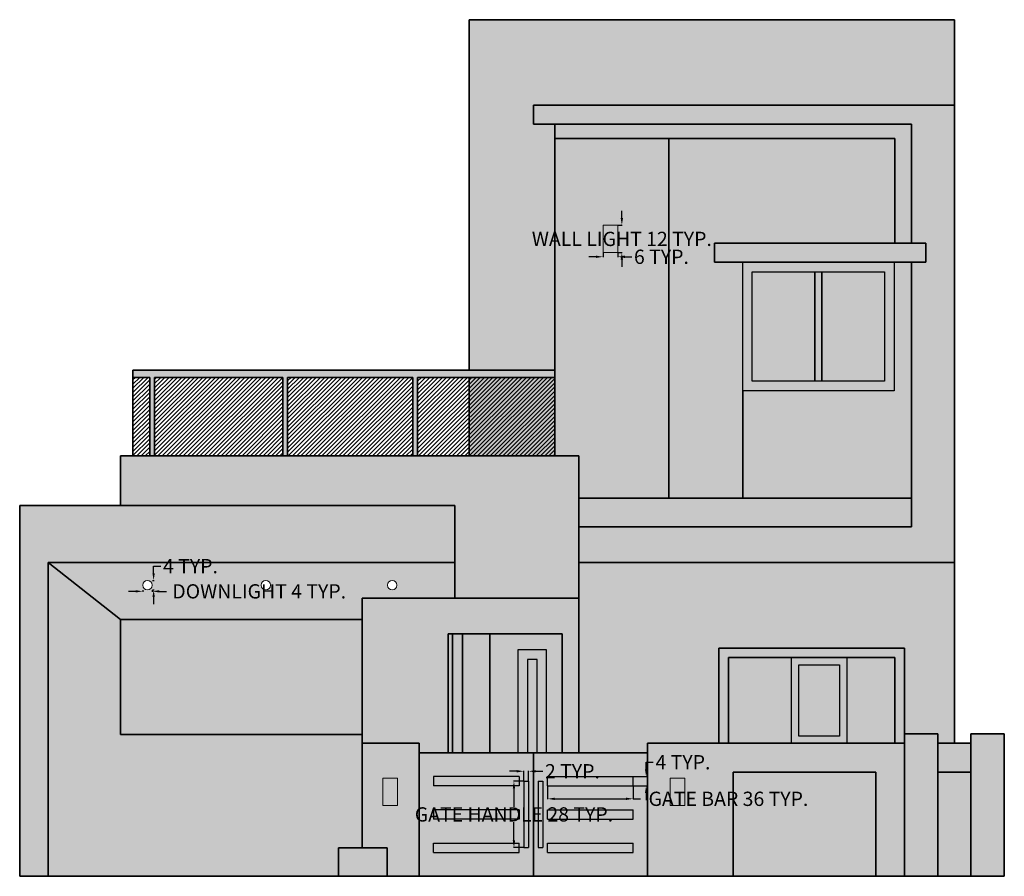
# Model space of a CAD drawing. Units: inches. Extents: x 25 to 439, y 12 to 373.
import ezdxf

# ---------------------------------------------------------------- set-up
doc = ezdxf.new("R2010")
doc.units = ezdxf.units.IN
doc.header["$MEASUREMENT"] = 0
for name, color, linetype, lineweight in [('A-ANNO-DIMS', 2, 'Continuous', 18), ('A-DOOR', 3, 'Continuous', 25), ('A-ELEV', 7, 'Continuous', 35), ('A-ELEV-PATT', 8, 'Continuous', 13), ('A-GLAZ', 4, 'Continuous', 25), ('E-LITE', 2, 'Continuous', 18)]:
    doc.layers.add(name, color=color, linetype=linetype, lineweight=lineweight)
doc.styles.get("Standard").update_dxf_attribs({"font": 'arial.ttf'})
doc.dimstyles.get("Standard").update_dxf_attribs({"dimtxt": 6, "dimasz": 3, "dimexe": 0.18, "dimexo": 0.0625, "dimgap": 0.09, "dimtad": 0, "dimtih": 1, "dimtoh": 1, "dimdec": 0, "dimzin": 0, "dimdsep": 46, "dimlunit": 3, "dimtxsty": 'Standard', "dimcen": 0.09, "dimadec": 0, "dimazin": 0, "dimtfac": 1, "dimtdec": 0, "dimtofl": 0, "dimtmove": 0, "dimatfit": 3, "dimfxl": 1, "dimtolj": 1, "dimtzin": 0, "dimarcsym": 0})

# ---------------------------------------------------------------- blocks, each defined once
blk = doc.blocks.new('GATE-BAR')
for p, q in [((0, 0), (0, 4)), ((0, 4), (36, 4)), ((36, 0), (36, 4)), ((0, 0), (36, 0))]:
    blk.add_line(p, q)
blk = doc.blocks.new('GATE-HANDLE')
for p, q in [((0, 27.93), (0, 0)), ((0, 27.93), (2, 27.93)), ((2, 27.93), (2, 0)), ((0, 0), (2, 0))]:
    blk.add_line(p, q)
blk = doc.blocks.new('WALL-LIGHT')
blk.add_lwpolyline([(0, 11.58), (6.15, 11.58), (6.15, 0), (0, 0)], close=True)
blk = doc.blocks.new('LIGHT-DOWN')
blk.add_circle((2, 2), 2)
blk = doc.blocks.new('*D5')
at = {"layer": 'A-ANNO-DIMS', "color": 0, "lineweight": -2, "transparency": 16777216}
for p, q in [((246.85, 50.12), (246.85, 44.6)), ((282.85, 50.12), (282.85, 44.6)), ((249.85, 44.78), (279.85, 44.78)), ((282.85, 44.78), (285.85, 44.78))]:
    blk.add_line(p, q, dxfattribs=at)
at = {"layer": 'A-ANNO-DIMS', "color": 0, "transparency": 16777216}
for points in [[(249.85, 45.28), (249.85, 44.28), (246.85, 44.78)], [(279.85, 45.28), (279.85, 44.28), (282.85, 44.78)]]:
    blk.add_solid(points, dxfattribs=at)
at = {"layer": 'Defpoints', "color": 0, "transparency": 16777216}
for p in [(246.85, 50.18), (282.85, 50.18), (282.85, 44.78)]:
    blk.add_point(p, dxfattribs=at)
at = {"layer": 'A-ANNO-DIMS', "color": 0, "transparency": 16777216, "insert": (322.86, 44.78), "char_height": 6, "attachment_point": 5}
blk.add_mtext('\\A1;GATE BAR 36 TYP.', dxfattribs=at)
blk = doc.blocks.new('*D6')
at = {"layer": 'A-ANNO-DIMS', "color": 0, "lineweight": -2, "transparency": 16777216}
for p, q in [((288.25, 57.18), (288.25, 60.18)), ((288.25, 60.18), (291.25, 60.18)), ((282.92, 54.18), (288.43, 54.18)), ((282.92, 50.18), (288.43, 50.18)), ((288.25, 47.18), (288.25, 44.18))]:
    blk.add_line(p, q, dxfattribs=at)
at = {"layer": 'A-ANNO-DIMS', "color": 0, "transparency": 16777216}
for points in [[(287.75, 57.18), (288.75, 57.18), (288.25, 54.18)], [(287.75, 47.18), (288.75, 47.18), (288.25, 50.18)]]:
    blk.add_solid(points, dxfattribs=at)
at = {"layer": 'Defpoints', "color": 0, "transparency": 16777216}
for p in [(282.85, 54.18), (288.25, 54.18), (282.85, 50.18)]:
    blk.add_point(p, dxfattribs=at)
at = {"layer": 'A-ANNO-DIMS', "color": 0, "transparency": 16777216, "insert": (303.74, 60.18), "char_height": 6, "attachment_point": 5}
blk.add_mtext('\\A1;4 TYP.', dxfattribs=at)
blk = doc.blocks.new('*D7')
at = {"layer": 'A-ANNO-DIMS', "color": 0, "lineweight": -2, "transparency": 16777216}
for p, q in [((278.04, 289.09), (278.04, 292.09)), ((276.37, 286.09), (278.22, 286.09)), ((276.37, 274.51), (278.22, 274.51)), ((278.04, 271.51), (278.04, 268.51))]:
    blk.add_line(p, q, dxfattribs=at)
at = {"layer": 'A-ANNO-DIMS', "color": 0, "transparency": 16777216}
for points in [[(277.54, 289.09), (278.54, 289.09), (278.04, 286.09)], [(277.54, 271.51), (278.54, 271.51), (278.04, 274.51)]]:
    blk.add_solid(points, dxfattribs=at)
at = {"layer": 'Defpoints', "color": 0, "transparency": 16777216}
for p in [(276.31, 286.09), (278.04, 286.09), (276.31, 274.51)]:
    blk.add_point(p, dxfattribs=at)
at = {"layer": 'A-ANNO-DIMS', "color": 0, "transparency": 16777216, "insert": (278.04, 280.3), "char_height": 6, "attachment_point": 5}
blk.add_mtext('\\A1;WALL LIGHT 12 TYP.', dxfattribs=at)
blk = doc.blocks.new('*D8')
at = {"layer": 'A-ANNO-DIMS', "color": 0, "lineweight": -2, "transparency": 16777216}
for p, q in [((270.16, 274.45), (270.16, 272.6)), ((276.31, 274.45), (276.31, 272.6)), ((267.16, 272.78), (264.16, 272.78)), ((279.31, 272.78), (282.31, 272.78))]:
    blk.add_line(p, q, dxfattribs=at)
at = {"layer": 'A-ANNO-DIMS', "color": 0, "transparency": 16777216}
for points in [[(267.16, 273.28), (267.16, 272.28), (270.16, 272.78)], [(279.31, 273.28), (279.31, 272.28), (276.31, 272.78)]]:
    blk.add_solid(points, dxfattribs=at)
at = {"layer": 'Defpoints', "color": 0, "transparency": 16777216}
for p in [(270.16, 274.51), (276.31, 274.51), (276.31, 272.78)]:
    blk.add_point(p, dxfattribs=at)
at = {"layer": 'A-ANNO-DIMS', "color": 0, "transparency": 16777216, "insert": (294.68, 272.78), "char_height": 6, "attachment_point": 5}
blk.add_mtext('\\A1;6 TYP.', dxfattribs=at)
blk = doc.blocks.new('*D9')
at = {"layer": 'A-ANNO-DIMS', "color": 0, "lineweight": -2, "transparency": 16777216}
for p, q in [((76.57, 132.59), (76.57, 131.87)), ((80.57, 132.59), (80.57, 131.87)), ((73.57, 132.05), (70.57, 132.05)), ((83.57, 132.05), (86.57, 132.05))]:
    blk.add_line(p, q, dxfattribs=at)
at = {"layer": 'A-ANNO-DIMS', "color": 0, "transparency": 16777216}
for points in [[(73.57, 132.55), (73.57, 131.55), (76.57, 132.05)], [(83.57, 132.55), (83.57, 131.55), (80.57, 132.05)]]:
    blk.add_solid(points, dxfattribs=at)
at = {"layer": 'Defpoints', "color": 0, "transparency": 16777216}
for p in [(76.57, 132.65), (80.57, 132.65), (80.57, 132.05)]:
    blk.add_point(p, dxfattribs=at)
at = {"layer": 'A-ANNO-DIMS', "color": 0, "transparency": 16777216, "insert": (125.56, 132.05), "char_height": 6, "attachment_point": 5}
blk.add_mtext('\\A1;DOWNLIGHT 4 TYP.', dxfattribs=at)
blk = doc.blocks.new('*D10')
at = {"layer": 'A-ANNO-DIMS', "color": 0, "lineweight": -2, "transparency": 16777216}
for p, q in [((81.17, 139.65), (81.17, 142.65)), ((81.17, 142.65), (84.17, 142.65)), ((80.63, 136.65), (81.35, 136.65)), ((80.63, 132.65), (81.35, 132.65)), ((81.17, 129.65), (81.17, 126.65))]:
    blk.add_line(p, q, dxfattribs=at)
at = {"layer": 'A-ANNO-DIMS', "color": 0, "transparency": 16777216}
for points in [[(80.67, 139.65), (81.67, 139.65), (81.17, 136.65)], [(80.67, 129.65), (81.67, 129.65), (81.17, 132.65)]]:
    blk.add_solid(points, dxfattribs=at)
at = {"layer": 'Defpoints', "color": 0, "transparency": 16777216}
for p in [(80.57, 136.65), (81.17, 136.65), (80.57, 132.65)]:
    blk.add_point(p, dxfattribs=at)
at = {"layer": 'A-ANNO-DIMS', "color": 0, "transparency": 16777216, "insert": (96.66, 142.65), "char_height": 6, "attachment_point": 5}
blk.add_mtext('\\A1;4 TYP.', dxfattribs=at)
blk = doc.blocks.new('*D11')
at = {"layer": 'A-ANNO-DIMS', "color": 0, "lineweight": -2, "transparency": 16777216}
for p, q in [((236.79, 52.18), (232.49, 52.18)), ((232.67, 49.18), (232.67, 41.41)), ((232.67, 27.25), (232.67, 35.02)), ((236.79, 24.25), (232.49, 24.25))]:
    blk.add_line(p, q, dxfattribs=at)
at = {"layer": 'A-ANNO-DIMS', "color": 0, "transparency": 16777216}
for points in [[(232.17, 49.18), (233.17, 49.18), (232.67, 52.18)], [(232.17, 27.25), (233.17, 27.25), (232.67, 24.25)]]:
    blk.add_solid(points, dxfattribs=at)
at = {"layer": 'Defpoints', "color": 0, "transparency": 16777216}
for p in [(232.67, 52.18), (236.85, 52.18), (236.85, 24.25)]:
    blk.add_point(p, dxfattribs=at)
at = {"layer": 'A-ANNO-DIMS', "color": 0, "transparency": 16777216, "insert": (232.67, 38.22), "char_height": 6, "attachment_point": 5}
blk.add_mtext('\\A1;GATE HANDLE 28 TYP.', dxfattribs=at)
blk = doc.blocks.new('*D12')
at = {"layer": 'A-ANNO-DIMS', "color": 0, "lineweight": -2, "transparency": 16777216}
for p, q in [((233.85, 56.37), (230.85, 56.37)), ((236.85, 52.24), (236.85, 56.55)), ((238.85, 52.24), (238.85, 56.55)), ((241.85, 56.37), (244.85, 56.37))]:
    blk.add_line(p, q, dxfattribs=at)
at = {"layer": 'A-ANNO-DIMS', "color": 0, "transparency": 16777216}
for points in [[(233.85, 56.87), (233.85, 55.87), (236.85, 56.37)], [(241.85, 56.87), (241.85, 55.87), (238.85, 56.37)]]:
    blk.add_solid(points, dxfattribs=at)
at = {"layer": 'Defpoints', "color": 0, "transparency": 16777216}
for p in [(238.85, 56.37), (236.85, 52.18), (238.85, 52.18)]:
    blk.add_point(p, dxfattribs=at)
at = {"layer": 'A-ANNO-DIMS', "color": 0, "transparency": 16777216, "insert": (257.27, 56.37), "char_height": 6, "attachment_point": 5}
blk.add_mtext('\\A1;2 TYP.', dxfattribs=at)

msp = doc.modelspace()

# ---------------------------------------------------------------- hatches: boundary and pattern name
at = {"layer": 'A-ELEV-PATT'}
h = msp.add_hatch(color=256, dxfattribs=at)
h.dxf.hatch_style = 1
h.paths.add_polyline_path([(417.85, 372.5), (213.85, 372.5), (213.85, 225.05), (249.85, 225.05), (249.85, 328.5), (240.85, 328.5), (240.85, 336.5), (249.85, 336.5), (417.85, 336.5)])
h.paths.add_polyline_path([(192.85, 68.18), (168.85, 68.18), (168.85, 24.18), (179.42, 24.18), (179.42, 12.18), (192.85, 12.18)])
h.paths.add_polyline_path([(183.68, 41.91), (177.53, 41.91), (177.53, 53.48), (183.68, 53.48)], flags=16)
h.paths.add_polyline_path([(324.85, 56.03), (384.85, 56.03), (384.85, 12.18), (396.85, 12.18), (396.85, 68.18), (288.85, 68.18), (288.85, 12.18), (324.85, 12.18)])
h.paths.add_polyline_path([(304.5, 41.91), (298.35, 41.91), (298.35, 53.48), (304.5, 53.48)], flags=16)
h = msp.add_hatch(color=256, dxfattribs=at)
h.dxf.hatch_style = 1
h.paths.add_polyline_path([(417.85, 336.5), (249.85, 336.5), (240.85, 336.5), (240.85, 328.5), (399.85, 328.5), (399.85, 278.5), (405.85, 278.5), (405.85, 270.5), (399.85, 270.5), (399.85, 159.18), (259.99, 159.18), (259.99, 144.18), (417.85, 144.18)])
h.paths.add_polyline_path([(405.85, 278.5), (399.85, 278.5), (392.85, 278.5), (316.94, 278.5), (316.94, 270.5), (340.85, 270.5), (392.5, 270.5), (393.85, 270.5), (399.85, 270.5), (405.85, 270.5)], flags=17)
h = msp.add_hatch(color=256, dxfattribs=at)
h.dxf.hatch_style = 1
h.paths.add_polyline_path([(399.85, 328.5), (249.85, 328.5), (249.85, 322.5), (399.85, 322.5)])
h.paths.add_polyline_path([(399.85, 322.5), (392.85, 322.5), (392.85, 278.5), (399.85, 278.5)])
h = msp.add_hatch(color=256, dxfattribs=at)
h.dxf.hatch_style = 1
h.paths.add_polyline_path([(297.85, 322.5), (249.85, 322.5), (249.85, 189.05), (259.99, 189.05), (259.99, 171.18), (297.85, 171.18)])
h.paths.add_polyline_path([(276.31, 274.51), (270.16, 274.51), (270.16, 286.09), (276.31, 286.09)], flags=16)
h = msp.add_hatch(color=256, dxfattribs=at)
h.dxf.hatch_style = 1
h.paths.add_polyline_path([(392.85, 322.5), (297.85, 322.5), (297.85, 171.18), (328.9, 171.18), (328.9, 216.41), (328.9, 270.5), (316.94, 270.5), (316.94, 278.5), (392.85, 278.5)])
h = msp.add_hatch(color=256, dxfattribs=at)
h.paths.add_polyline_path([(288.85, 64.18), (240.85, 64.18), (240.85, 12.18), (288.85, 12.18)])
h.paths.add_polyline_path([(282.85, 54.18), (282.85, 50.18), (246.85, 50.18), (246.85, 54.18)], flags=16)
h.paths.add_polyline_path([(244.81, 52.18), (244.81, 24.25), (242.81, 24.25), (242.81, 52.18)], flags=16)
h.paths.add_polyline_path([(282.85, 40.18), (282.85, 36.18), (246.85, 36.18), (246.85, 40.18)], flags=16)
h.paths.add_polyline_path([(282.85, 26.18), (282.85, 22.18), (246.85, 22.18), (246.85, 26.18)], flags=16)
h.paths.add_polyline_path([(240.85, 64.18), (238.35, 64.18), (234.27, 64.18), (192.85, 64.18), (192.85, 12.18), (240.85, 12.18)])
h.paths.add_polyline_path([(234.85, 54.18), (234.85, 50.18), (198.85, 50.18), (198.85, 54.18)], flags=16)
h.paths.add_polyline_path([(236.85, 52.18), (238.85, 52.18), (238.85, 24.25), (236.85, 24.25)], flags=16)
h.paths.add_polyline_path([(234.85, 40.18), (234.85, 36.18), (198.85, 36.18), (198.85, 40.18)], flags=16)
h.paths.add_polyline_path([(234.85, 26.18), (234.85, 22.18), (198.85, 22.18), (198.85, 26.18)], flags=16)
h.paths.add_polyline_path([(304.5, 53.48), (298.35, 53.48), (298.35, 41.91), (304.5, 41.91)])
h.paths.add_polyline_path([(183.68, 53.48), (177.53, 53.48), (177.53, 41.91), (183.68, 41.91)])
h.paths.add_polyline_path([(276.31, 286.09), (270.16, 286.09), (270.16, 274.51), (276.31, 274.51)])
h = msp.add_hatch(color=256, dxfattribs=at)
h.dxf.hatch_style = 1
h.paths.add_polyline_path([(399.85, 270.5), (393.85, 270.5), (392.5, 270.5), (392.5, 216.41), (328.9, 216.41), (328.9, 171.18), (399.85, 171.18)])
h.paths.add_polyline_path([(168.85, 129.18), (207.85, 129.18), (207.85, 144.18), (36.85, 144.18), (67.2, 120.18), (168.85, 120.18)])
h.paths.add_polyline_path([(76.57, 134.65, -1), (80.57, 134.65, -1)], flags=16)
h.paths.add_polyline_path([(126.34, 134.65, -1), (130.34, 134.65, -1)], flags=16)
h.paths.add_polyline_path([(183.5, 134.65, -1), (179.5, 134.65, -1)], flags=16)
h = msp.add_hatch(color=256, dxfattribs=at)
h.paths.add_polyline_path([(396.85, 108.18), (318.85, 108.18), (318.85, 68.18), (322.85, 68.18), (322.85, 104.18), (392.85, 104.18), (392.85, 68.18), (396.85, 68.18), (396.85, 72.18)])
h.paths.add_polyline_path([(372.58, 104.18), (349.4, 104.18), (349.4, 68.18), (372.58, 68.18)], flags=17)
h.paths.add_polyline_path([(369.58, 101.18), (369.58, 71.18), (352.4, 71.18), (352.4, 101.18)], flags=16)
h.paths.add_polyline_path([(392.5, 270.5), (328.9, 270.5), (328.9, 216.41), (392.5, 216.41)])
h.paths.add_polyline_path([(388.5, 266.5), (388.5, 220.41), (332.9, 220.41), (332.9, 266.5)], flags=16)
h = msp.add_hatch(color=256, dxfattribs=at)
h.set_gradient(color1=(254, 204, 102), name='CYLINDER')
h.paths.add_polyline_path([(332.9, 220.41), (359.2, 220.41), (359.2, 266.5), (332.9, 266.5)])
for points in [[(362.2, 266.5), (359.2, 266.5), (359.2, 220.41), (362.2, 220.41)], [(249.85, 225.05), (72.49, 225.05), (72.49, 222.05), (79.55, 222.05), (79.55, 189.05), (81.55, 189.05), (81.55, 222.05), (135.52, 222.05), (135.52, 189.05), (137.52, 189.05), (137.52, 222.05), (190.12, 222.05), (190.12, 189.05), (192.12, 189.05), (192.12, 222.05), (249.85, 222.05)], [(249.85, 222.05), (213.85, 222.05), (213.85, 189.05), (249.85, 189.05)], [(168.85, 120.18), (67.2, 120.18), (67.2, 71.77), (168.85, 71.77)], [(242.46, 103.31), (238.35, 103.31), (238.35, 64.18), (242.46, 64.18)], [(424.85, 56.03), (410.85, 56.03), (410.85, 12.18), (424.85, 12.18)]]:
    msp.add_hatch(color=256, dxfattribs=at).paths.add_polyline_path(points)
h = msp.add_hatch(color=256, dxfattribs=at)
h.set_gradient(color1=(254, 204, 102), name='CYLINDER')
h.paths.add_polyline_path([(388.5, 266.5), (362.2, 266.5), (362.2, 220.41), (388.5, 220.41)])
h = msp.add_hatch(dxfattribs=at)
h.set_pattern_fill('ANSI31', color=256, scale=10, style=0)
h.paths.add_polyline_path([(135.52, 222.05), (81.55, 222.05), (81.55, 189.05), (135.52, 189.05)])
h.paths.add_polyline_path([(79.55, 222.05), (72.49, 222.05), (72.49, 189.05), (79.55, 189.05)])
h.paths.add_polyline_path([(190.12, 222.05), (137.52, 222.05), (137.52, 189.05), (190.12, 189.05)])
h.paths.add_polyline_path([(213.85, 222.05), (192.12, 222.05), (192.12, 189.05), (213.85, 189.05)])
h.paths.add_polyline_path([(249.85, 222.05), (213.85, 222.05), (213.85, 189.05), (249.85, 189.05)])
h = msp.add_hatch(color=256, dxfattribs=at)
h.dxf.hatch_style = 1
h.paths.add_polyline_path([(259.99, 189.05), (67.2, 189.05), (67.2, 168.18), (207.85, 168.18), (207.85, 129.18), (259.99, 129.18), (259.99, 171.18)])
h.paths.add_polyline_path([(384.85, 56.03), (324.85, 56.03), (324.85, 12.18), (384.85, 12.18)])
h.paths.add_polyline_path([(318.85, 108.18), (396.85, 108.18), (396.85, 72.18), (410.85, 72.18), (410.85, 68.18), (417.85, 68.18), (417.85, 120.18), (259.99, 120.18), (259.99, 64.18), (288.85, 64.18), (288.85, 68.18), (318.85, 68.18)])
h.paths.add_polyline_path([(417.85, 144.18), (259.99, 144.18), (259.99, 129.18), (259.99, 120.18), (417.85, 120.18)])
h = msp.add_hatch(color=256, dxfattribs=at)
h.dxf.hatch_style = 1
h.paths.add_polyline_path([(179.42, 24.18), (158.92, 24.18), (158.92, 12.18), (179.42, 12.18)])
h.paths.add_polyline_path([(424.85, 68.18), (410.85, 68.18), (410.85, 56.03), (424.85, 56.03)])
h.paths.add_polyline_path([(399.85, 171.18), (259.99, 171.18), (259.99, 159.18), (399.85, 159.18)])
h = msp.add_hatch(color=256, dxfattribs=at)
h.dxf.hatch_style = 1
h.paths.add_polyline_path([(207.85, 168.18), (24.85, 168.18), (24.85, 12.18), (36.85, 12.18), (36.85, 144.18), (207.85, 144.18)])
h = msp.add_hatch(color=256, dxfattribs=at)
h.set_gradient(color1=(248, 246, 176), name='CYLINDER')
h.paths.add_polyline_path([(158.92, 12.18), (158.92, 24.18), (168.85, 24.18), (168.85, 71.77), (67.2, 71.77), (67.2, 120.18), (36.85, 144.18), (36.85, 12.18)])
h = msp.add_hatch(color=256, dxfattribs=at)
h.set_gradient(color1=(248, 246, 176), name='CYLINDER')
h.paths.add_polyline_path([(168.85, 68.18), (192.85, 68.18), (192.85, 64.18), (204.99, 64.18), (204.99, 114.15), (252.99, 114.15), (252.99, 64.18), (259.99, 64.18), (259.99, 129.18), (168.85, 129.18), (168.85, 120.18)])
h = msp.add_hatch(color=256, dxfattribs=at)
h.paths.add_polyline_path([(252.99, 114.15), (222.49, 114.15), (222.49, 64.18), (234.27, 64.18), (234.27, 107.38), (246.39, 107.38), (246.39, 64.18), (252.99, 64.18)])
h.paths.add_polyline_path([(222.49, 114.15), (210.99, 114.15), (210.99, 64.18), (222.49, 64.18)])
h.paths.add_polyline_path([(210.99, 114.15), (206.81, 114.15), (206.81, 64.18), (210.99, 64.18)])
h.paths.add_polyline_path([(206.81, 114.15), (204.99, 114.15), (204.99, 64.18), (206.81, 64.18)])
h.paths.add_polyline_path([(238.35, 103.31), (242.46, 103.31), (242.46, 64.18), (246.39, 64.18), (246.39, 107.38), (234.27, 107.38), (234.27, 64.18), (238.35, 64.18)], flags=17)
h = msp.add_hatch(color=256, dxfattribs=at)
h.set_gradient(color1=(254, 204, 102), name='CYLINDER')
h.paths.add_polyline_path([(349.4, 104.18), (322.85, 104.18), (322.85, 68.18), (349.4, 68.18)])
h = msp.add_hatch(color=256, dxfattribs=at)
h.set_gradient(color1=(254, 204, 102), name='CYLINDER')
h.paths.add_polyline_path([(392.85, 104.18), (372.58, 104.18), (372.58, 68.18), (392.85, 68.18)])
h = msp.add_hatch(color=256, dxfattribs=at)
h.set_gradient(color1=(254, 204, 102), name='CYLINDER')
h.paths.add_polyline_path([(352.4, 71.18), (369.58, 71.18), (369.58, 101.18), (352.4, 101.18)])
h = msp.add_hatch(color=256, dxfattribs=at)
h.paths.add_polyline_path([(438.85, 72.18), (424.85, 72.18), (424.85, 12.18), (438.85, 12.18)])
h.paths.add_polyline_path([(410.85, 72.18), (396.85, 72.18), (396.85, 12.18), (410.85, 12.18)])
h = msp.add_hatch(color=256, dxfattribs=at)
h.paths.add_polyline_path([(282.85, 54.18), (246.85, 54.18), (246.85, 50.18), (282.85, 50.18)])
h.paths.add_polyline_path([(234.85, 54.18), (198.85, 54.18), (198.85, 50.18), (234.85, 50.18)])
h.paths.add_polyline_path([(234.85, 40.18), (198.85, 40.18), (198.85, 36.18), (234.85, 36.18)])
h.paths.add_polyline_path([(234.85, 26.18), (198.85, 26.18), (198.85, 22.18), (234.85, 22.18)])
h.paths.add_polyline_path([(282.85, 26.18), (246.85, 26.18), (246.85, 22.18), (282.85, 22.18)])
h.paths.add_polyline_path([(282.85, 40.18), (246.85, 40.18), (246.85, 36.18), (282.85, 36.18)])
h = msp.add_hatch(color=256, dxfattribs=at)
h.paths.add_polyline_path([(238.85, 52.18), (236.85, 52.18), (236.85, 24.25), (238.85, 24.25)])
h.paths.add_polyline_path([(244.81, 52.18), (242.81, 52.18), (242.81, 24.25), (244.81, 24.25)])

# ---------------------------------------------------------------- linework, layer by layer
at = {"layer": 'A-DOOR'}
for points in [[(246.39, 107.38), (234.27, 107.38), (234.27, 64.18), (246.39, 64.18)], [(242.46, 103.31), (238.35, 103.31), (238.35, 64.18), (242.46, 64.18)]]:
    msp.add_lwpolyline(points, close=True, dxfattribs=at)
at = {"layer": 'A-ELEV'}
for p, q in [((417.85, 372.5), (213.85, 372.5)), ((213.85, 372.5), (213.85, 225.05)), ((417.85, 68.18), (417.85, 372.5)), ((249.85, 336.5), (240.85, 336.5)), ((240.85, 336.5), (240.85, 328.5)), ((417.85, 336.5), (249.85, 336.5)), ((240.85, 328.5), (399.85, 328.5)), ((249.85, 328.5), (249.85, 189.05)), ((399.85, 278.5), (399.85, 328.5)), ((249.85, 322.5), (392.85, 322.5)), ((297.85, 322.5), (297.85, 171.18)), ((392.85, 322.5), (392.85, 278.5)), ((392.85, 278.5), (316.94, 278.5)), ((316.94, 278.5), (316.94, 270.5)), ((392.85, 278.5), (399.85, 278.5)), ((399.85, 278.5), (405.85, 278.5)), ((405.85, 278.5), (405.85, 270.5)), ((316.94, 270.5), (340.85, 270.5)), ((340.85, 270.5), (393.85, 270.5)), ((393.85, 270.5), (399.85, 270.5)), ((399.85, 159.18), (399.85, 270.5)), ((405.85, 270.5), (399.85, 270.5)), ((359.2, 266.5), (359.2, 220.41)), ((362.2, 266.5), (362.2, 220.41)), ((72.49, 189.05), (72.49, 225.05)), ((72.49, 225.05), (249.85, 225.05)), ((72.49, 222.05), (79.55, 222.05)), ((79.55, 189.05), (79.55, 222.05)), ((81.55, 189.05), (81.55, 222.05)), ((81.55, 222.05), (135.52, 222.05)), ((135.52, 189.05), (135.52, 222.05)), ((137.52, 189.05), (137.52, 222.05)), ((137.52, 222.05), (190.12, 222.05)), ((190.12, 189.05), (190.12, 222.05)), ((192.12, 189.05), (192.12, 222.05)), ((192.12, 222.05), (249.85, 222.05)), ((213.85, 222.05), (213.85, 189.05)), ((328.9, 216.41), (328.9, 171.18)), ((259.99, 189.05), (67.2, 189.05)), ((67.2, 168.18), (67.2, 189.05)), ((259.99, 171.18), (259.99, 189.05)), ((259.99, 171.18), (399.85, 171.18)), ((259.99, 64.18), (259.99, 171.18)), ((24.85, 12.18), (24.85, 168.18)), ((24.85, 168.18), (207.85, 168.18)), ((207.85, 168.18), (207.85, 129.18)), ((259.99, 159.18), (399.85, 159.18)), ((36.85, 12.18), (36.85, 144.18)), ((36.85, 144.18), (207.85, 144.18)), ((36.85, 144.18), (67.2, 120.18)), ((259.99, 144.18), (417.85, 144.18)), ((168.85, 120.18), (168.85, 129.18)), ((168.85, 129.18), (259.99, 129.18)), ((67.2, 71.77), (67.2, 120.18)), ((67.2, 120.18), (168.85, 120.18)), ((168.85, 24.18), (168.85, 120.18)), ((204.99, 64.18), (204.99, 114.15)), ((204.99, 114.15), (252.99, 114.15)), ((206.81, 64.18), (206.81, 114.15)), ((210.99, 64.18), (210.99, 114.15)), ((222.49, 114.15), (222.49, 64.18)), ((252.99, 64.18), (252.99, 114.15)), ((396.85, 108.18), (318.85, 108.18)), ((318.85, 108.18), (318.85, 68.18)), ((396.85, 72.18), (396.85, 108.18)), ((392.85, 104.18), (322.85, 104.18)), ((322.85, 104.18), (322.85, 68.18)), ((392.85, 68.18), (392.85, 104.18)), ((67.2, 71.77), (168.85, 71.77)), ((396.85, 12.18), (396.85, 72.18)), ((396.85, 72.18), (410.85, 72.18)), ((410.85, 12.18), (410.85, 72.18)), ((424.85, 12.18), (424.85, 72.18)), ((424.85, 72.18), (438.85, 72.18)), ((438.85, 12.18), (438.85, 72.18)), ((168.85, 68.18), (192.85, 68.18)), ((192.85, 12.18), (192.85, 68.18)), ((288.85, 12.18), (288.85, 68.18)), ((288.85, 68.18), (396.85, 68.18)), ((410.85, 68.18), (424.85, 68.18)), ((192.85, 64.18), (288.85, 64.18)), ((240.85, 12.18), (240.85, 64.18)), ((324.85, 56.03), (384.85, 56.03)), ((324.85, 12.18), (324.85, 56.03)), ((384.85, 12.18), (384.85, 56.03)), ((410.85, 56.03), (424.85, 56.03)), ((179.42, 24.18), (158.92, 24.18)), ((158.92, 24.18), (158.92, 12.18)), ((179.42, 12.18), (179.42, 24.18)), ((24.85, 12.18), (438.85, 12.18))]:
    msp.add_line(p, q, dxfattribs=at)
at = {"layer": 'A-GLAZ'}
for points in [[(328.9, 270.5), (392.5, 270.5), (392.5, 216.41), (328.9, 216.41)], [(332.9, 266.5), (388.5, 266.5), (388.5, 220.41), (332.9, 220.41)], [(349.4, 104.18), (372.58, 104.18), (372.58, 68.18), (349.4, 68.18)], [(352.4, 101.18), (369.58, 101.18), (369.58, 71.18), (352.4, 71.18)]]:
    msp.add_lwpolyline(points, close=True, dxfattribs=at)

# ---------------------------------------------------------------- block references
at = {"layer": 'A-DOOR', "rotation": 180}
for p in [(234.85, 54.18), (234.85, 40.18)]:
    msp.add_blockref('GATE-BAR', p, dxfattribs=at)
at = {"layer": 'A-DOOR'}
for name, p in [('GATE-BAR', (246.85, 50.18)), ('GATE-HANDLE', (236.85, 24.25)), ('GATE-HANDLE', (242.81, 24.25)), ('GATE-BAR', (246.85, 36.18)), ('GATE-BAR', (198.85, 22.18)), ('GATE-BAR', (246.85, 22.18))]:
    msp.add_blockref(name, p, dxfattribs=at)
at = {"layer": 'E-LITE'}
for name, p in [('WALL-LIGHT', (270.16, 274.51)), ('LIGHT-DOWN', (76.57, 132.65)), ('LIGHT-DOWN', (126.34, 132.65)), ('LIGHT-DOWN', (179.5, 132.65)), ('WALL-LIGHT', (177.53, 41.91)), ('WALL-LIGHT', (298.35, 41.91))]:
    msp.add_blockref(name, p, dxfattribs=at)

# ---------------------------------------------------------------- dimensions: what is measured, and where the dimension line sits
at = {"layer": 'A-ANNO-DIMS'}
for base, p1, p2, text, picture, middle in [((278.04, 286.09), (276.31, 274.51), (276.31, 286.09), 'WALL LIGHT <> TYP.', '*D7', (278.04, 280.3)), ((81.17, 136.65), (80.57, 132.65), (80.57, 136.65), '<> TYP.', '*D10', (96.66, 142.65)), ((288.25, 54.18), (282.85, 50.18), (282.85, 54.18), '<> TYP.', '*D6', (303.74, 60.18)), ((232.67, 52.18), (236.85, 24.25), (236.85, 52.18), 'GATE HANDLE <> TYP.', '*D11', (232.67, 38.22))]:
    dim = msp.add_linear_dim(base=base, p1=p1, p2=p2, angle=90, text=text, dimstyle='Standard', override={"dimdec": 0, "dimlfac": 1, "dimrnd": 0, "dimzin": 0, "dimdsep": 46, "dimlunit": 2}, dxfattribs=at)
    dim.commit()
    dim.dimension.update_dxf_attribs({"geometry": picture, "text_midpoint": middle})
for base, p1, p2, text, picture, middle in [((276.31, 272.78), (270.16, 274.51), (276.31, 274.51), '<> TYP.', '*D8', (294.68, 272.78)), ((80.57, 132.05), (76.57, 132.65), (80.57, 132.65), 'DOWNLIGHT <> TYP.', '*D9', (125.56, 132.05)), ((238.85, 56.37), (236.85, 52.18), (238.85, 52.18), '<> TYP.', '*D12', (257.27, 56.37)), ((282.85, 44.78), (246.85, 50.18), (282.85, 50.18), 'GATE BAR <> TYP.', '*D5', (322.86, 44.78))]:
    dim = msp.add_linear_dim(base=base, p1=p1, p2=p2, text=text, dimstyle='Standard', override={"dimdec": 0, "dimlfac": 1, "dimrnd": 0, "dimzin": 0, "dimdsep": 46, "dimlunit": 2}, dxfattribs=at)
    dim.commit()
    dim.dimension.update_dxf_attribs({"geometry": picture, "text_midpoint": middle})

doc.saveas('drawing.dxf')
